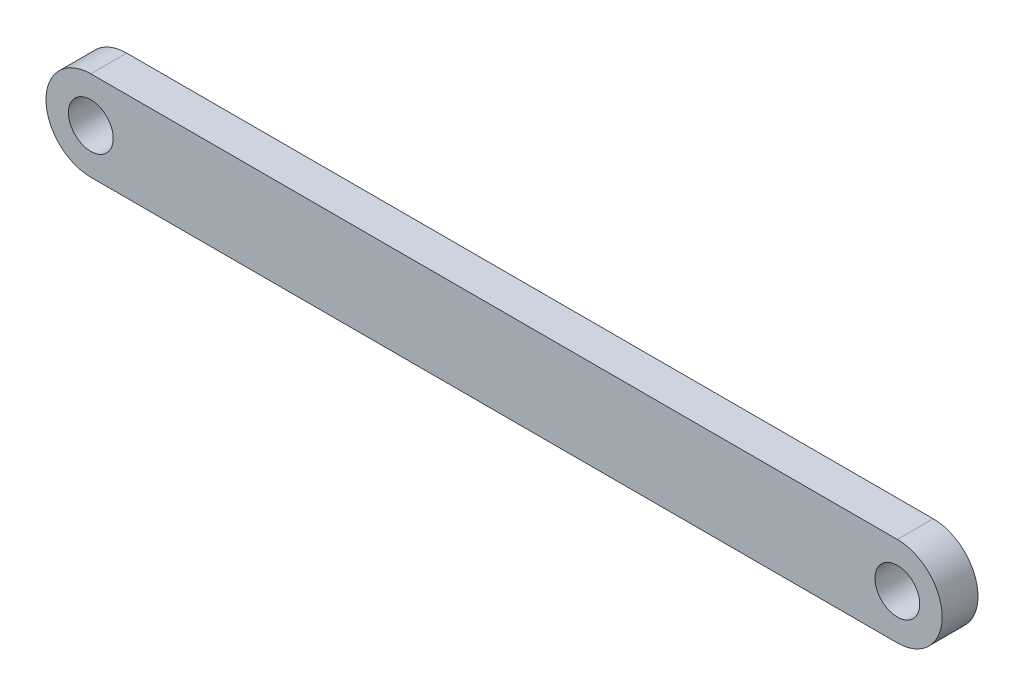
ISO-10303-21;
HEADER;
FILE_DESCRIPTION(('STEP AP214'),'2;1');
FILE_NAME('part.step','',(''),(''),'','','');
FILE_SCHEMA(('AUTOMOTIVE_DESIGN { 1 0 10303 214 1 1 1 1 }'));
ENDSEC;
DATA;
#1=APPLICATION_CONTEXT('core data for automotive mechanical design processes');
#2=APPLICATION_PROTOCOL_DEFINITION('international standard','automotive_design',2000,#1);
#3=PRODUCT_CONTEXT('',#1,'mechanical');
#4=PRODUCT('Part','Part','',(#3));
#5=PRODUCT_RELATED_PRODUCT_CATEGORY('part','',(#4));
#6=PRODUCT_DEFINITION_FORMATION('','',#4);
#7=PRODUCT_DEFINITION_CONTEXT('part definition',#1,'design');
#8=PRODUCT_DEFINITION('design','',#6,#7);
#9=PRODUCT_DEFINITION_SHAPE('','',#8);
#10=(LENGTH_UNIT() NAMED_UNIT(*) SI_UNIT(.MILLI.,.METRE.));
#11=(NAMED_UNIT(*) PLANE_ANGLE_UNIT() SI_UNIT($,.RADIAN.));
#12=(NAMED_UNIT(*) SI_UNIT($,.STERADIAN.) SOLID_ANGLE_UNIT());
#13=UNCERTAINTY_MEASURE_WITH_UNIT(LENGTH_MEASURE(1.E-05),#10,'distance_accuracy_value','');
#14=(GEOMETRIC_REPRESENTATION_CONTEXT(3) GLOBAL_UNCERTAINTY_ASSIGNED_CONTEXT((#13)) GLOBAL_UNIT_ASSIGNED_CONTEXT((#10,
#11,#12)) REPRESENTATION_CONTEXT('',''));
#15=CARTESIAN_POINT('',(0.,0.,0.));
#16=DIRECTION('',(0.,0.,1.));
#17=DIRECTION('',(1.,0.,0.));
#18=AXIS2_PLACEMENT_3D('',#15,#16,#17);
#19=CARTESIAN_POINT('',(-45.,0.,2.));
#20=DIRECTION('',(0.,0.,1.));
#21=DIRECTION('',(1.,0.,0.));
#22=AXIS2_PLACEMENT_3D('',#19,#20,#21);
#23=PLANE('',#22);
#24=CARTESIAN_POINT('',(-45.,0.,2.));
#25=DIRECTION('',(0.,0.,1.));
#26=DIRECTION('',(1.,0.,0.));
#27=AXIS2_PLACEMENT_3D('',#24,#25,#26);
#28=CIRCLE('',#27,2.5);
#29=CARTESIAN_POINT('',(-42.5,0.,2.));
#30=VERTEX_POINT('',#29);
#31=EDGE_CURVE('E106',#30,#30,#28,.T.);
#32=ORIENTED_EDGE('',*,*,#31,.F.);
#33=EDGE_LOOP('',(#32));
#34=FACE_BOUND('',#33,.T.);
#35=CARTESIAN_POINT('',(-45.,0.,2.));
#36=DIRECTION('',(0.,0.,1.));
#37=DIRECTION('',(1.,0.,0.));
#38=AXIS2_PLACEMENT_3D('',#35,#36,#37);
#39=CIRCLE('',#38,5.);
#40=CARTESIAN_POINT('',(-45.,5.,2.));
#41=VERTEX_POINT('',#40);
#42=CARTESIAN_POINT('',(-45.,-5.,2.));
#43=VERTEX_POINT('',#42);
#44=EDGE_CURVE('E93',#41,#43,#39,.T.);
#45=ORIENTED_EDGE('',*,*,#44,.T.);
#46=DIRECTION('',(1.,0.,0.));
#47=VECTOR('',#46,1.);
#48=CARTESIAN_POINT('',(-45.,-5.,2.));
#49=LINE('',#48,#47);
#50=CARTESIAN_POINT('',(45.,-5.,2.));
#51=VERTEX_POINT('',#50);
#52=EDGE_CURVE('E88',#43,#51,#49,.T.);
#53=ORIENTED_EDGE('',*,*,#52,.T.);
#54=CARTESIAN_POINT('',(45.,0.,2.));
#55=DIRECTION('',(0.,0.,1.));
#56=DIRECTION('',(1.,0.,0.));
#57=AXIS2_PLACEMENT_3D('',#54,#55,#56);
#58=CIRCLE('',#57,5.);
#59=CARTESIAN_POINT('',(45.,5.00000000000002,2.));
#60=VERTEX_POINT('',#59);
#61=EDGE_CURVE('E90',#51,#60,#58,.T.);
#62=ORIENTED_EDGE('',*,*,#61,.T.);
#63=DIRECTION('',(-1.,0.,0.));
#64=VECTOR('',#63,1.);
#65=CARTESIAN_POINT('',(-45.,5.,2.));
#66=LINE('',#65,#64);
#67=EDGE_CURVE('E57',#60,#41,#66,.T.);
#68=ORIENTED_EDGE('',*,*,#67,.T.);
#69=EDGE_LOOP('',(#45,#53,#62,#68));
#70=FACE_BOUND('',#69,.T.);
#71=CARTESIAN_POINT('',(45.,0.,2.));
#72=DIRECTION('',(0.,0.,1.));
#73=DIRECTION('',(1.,0.,0.));
#74=AXIS2_PLACEMENT_3D('',#71,#72,#73);
#75=CIRCLE('',#74,2.5);
#76=CARTESIAN_POINT('',(47.5,0.,2.));
#77=VERTEX_POINT('',#76);
#78=EDGE_CURVE('E122',#77,#77,#75,.T.);
#79=ORIENTED_EDGE('',*,*,#78,.F.);
#80=EDGE_LOOP('',(#79));
#81=FACE_BOUND('',#80,.T.);
#82=ADVANCED_FACE('F39',(#34,#70,#81),#23,.T.);
#83=CARTESIAN_POINT('',(-45.,0.,-2.));
#84=DIRECTION('',(0.,0.,1.));
#85=DIRECTION('',(1.,0.,0.));
#86=AXIS2_PLACEMENT_3D('',#83,#84,#85);
#87=PLANE('',#86);
#88=CARTESIAN_POINT('',(-45.,0.,-2.));
#89=DIRECTION('',(0.,0.,1.));
#90=DIRECTION('',(1.,0.,0.));
#91=AXIS2_PLACEMENT_3D('',#88,#89,#90);
#92=CIRCLE('',#91,5.);
#93=CARTESIAN_POINT('',(-45.,5.,-2.));
#94=VERTEX_POINT('',#93);
#95=CARTESIAN_POINT('',(-45.,-5.,-2.));
#96=VERTEX_POINT('',#95);
#97=EDGE_CURVE('E103',#94,#96,#92,.T.);
#98=ORIENTED_EDGE('',*,*,#97,.F.);
#99=DIRECTION('',(-1.,0.,0.));
#100=VECTOR('',#99,1.);
#101=CARTESIAN_POINT('',(-45.,5.,-2.));
#102=LINE('',#101,#100);
#103=CARTESIAN_POINT('',(45.,5.00000000000002,-2.));
#104=VERTEX_POINT('',#103);
#105=EDGE_CURVE('E76',#104,#94,#102,.T.);
#106=ORIENTED_EDGE('',*,*,#105,.F.);
#107=CARTESIAN_POINT('',(45.,0.,-2.));
#108=DIRECTION('',(0.,0.,1.));
#109=DIRECTION('',(1.,0.,0.));
#110=AXIS2_PLACEMENT_3D('',#107,#108,#109);
#111=CIRCLE('',#110,5.);
#112=CARTESIAN_POINT('',(45.,-5.,-2.));
#113=VERTEX_POINT('',#112);
#114=EDGE_CURVE('E71',#113,#104,#111,.T.);
#115=ORIENTED_EDGE('',*,*,#114,.F.);
#116=DIRECTION('',(1.,0.,0.));
#117=VECTOR('',#116,1.);
#118=CARTESIAN_POINT('',(-45.,-5.,-2.));
#119=LINE('',#118,#117);
#120=EDGE_CURVE('E92',#96,#113,#119,.T.);
#121=ORIENTED_EDGE('',*,*,#120,.F.);
#122=EDGE_LOOP('',(#98,#106,#115,#121));
#123=FACE_BOUND('',#122,.T.);
#124=CARTESIAN_POINT('',(-45.,0.,-2.));
#125=DIRECTION('',(0.,0.,1.));
#126=DIRECTION('',(1.,0.,0.));
#127=AXIS2_PLACEMENT_3D('',#124,#125,#126);
#128=CIRCLE('',#127,2.5);
#129=CARTESIAN_POINT('',(-42.5,0.,-2.));
#130=VERTEX_POINT('',#129);
#131=EDGE_CURVE('E119',#130,#130,#128,.T.);
#132=ORIENTED_EDGE('',*,*,#131,.T.);
#133=EDGE_LOOP('',(#132));
#134=FACE_BOUND('',#133,.T.);
#135=CARTESIAN_POINT('',(45.,0.,-2.));
#136=DIRECTION('',(0.,0.,1.));
#137=DIRECTION('',(1.,0.,0.));
#138=AXIS2_PLACEMENT_3D('',#135,#136,#137);
#139=CIRCLE('',#138,2.5);
#140=CARTESIAN_POINT('',(47.5,0.,-2.));
#141=VERTEX_POINT('',#140);
#142=EDGE_CURVE('E121',#141,#141,#139,.T.);
#143=ORIENTED_EDGE('',*,*,#142,.T.);
#144=EDGE_LOOP('',(#143));
#145=FACE_BOUND('',#144,.T.);
#146=ADVANCED_FACE('F111',(#123,#134,#145),#87,.F.);
#147=CARTESIAN_POINT('',(-45.,0.,2.));
#148=DIRECTION('',(0.,0.,-1.));
#149=DIRECTION('',(-1.,0.,0.));
#150=AXIS2_PLACEMENT_3D('',#147,#148,#149);
#151=CYLINDRICAL_SURFACE('',#150,5.);
#152=ORIENTED_EDGE('',*,*,#97,.T.);
#153=DIRECTION('',(0.,0.,-1.));
#154=VECTOR('',#153,1.);
#155=CARTESIAN_POINT('',(-45.,-5.,2.));
#156=LINE('',#155,#154);
#157=EDGE_CURVE('E11',#43,#96,#156,.T.);
#158=ORIENTED_EDGE('',*,*,#157,.F.);
#159=ORIENTED_EDGE('',*,*,#44,.F.);
#160=DIRECTION('',(0.,0.,-1.));
#161=VECTOR('',#160,1.);
#162=CARTESIAN_POINT('',(-45.,5.,2.));
#163=LINE('',#162,#161);
#164=EDGE_CURVE('E97',#41,#94,#163,.T.);
#165=ORIENTED_EDGE('',*,*,#164,.T.);
#166=EDGE_LOOP('',(#152,#158,#159,#165));
#167=FACE_BOUND('',#166,.T.);
#168=ADVANCED_FACE('F41',(#167),#151,.T.);
#169=CARTESIAN_POINT('',(-45.,-5.,2.));
#170=DIRECTION('',(0.,1.,0.));
#171=DIRECTION('',(-1.,0.,0.));
#172=AXIS2_PLACEMENT_3D('',#169,#170,#171);
#173=PLANE('',#172);
#174=ORIENTED_EDGE('',*,*,#120,.T.);
#175=DIRECTION('',(0.,0.,-1.));
#176=VECTOR('',#175,1.);
#177=CARTESIAN_POINT('',(45.,-5.,2.));
#178=LINE('',#177,#176);
#179=EDGE_CURVE('E48',#51,#113,#178,.T.);
#180=ORIENTED_EDGE('',*,*,#179,.F.);
#181=ORIENTED_EDGE('',*,*,#52,.F.);
#182=ORIENTED_EDGE('',*,*,#157,.T.);
#183=EDGE_LOOP('',(#174,#180,#181,#182));
#184=FACE_BOUND('',#183,.T.);
#185=ADVANCED_FACE('F94',(#184),#173,.F.);
#186=CARTESIAN_POINT('',(45.,0.,2.));
#187=DIRECTION('',(0.,0.,-1.));
#188=DIRECTION('',(-1.,0.,0.));
#189=AXIS2_PLACEMENT_3D('',#186,#187,#188);
#190=CYLINDRICAL_SURFACE('',#189,5.);
#191=ORIENTED_EDGE('',*,*,#114,.T.);
#192=DIRECTION('',(0.,0.,-1.));
#193=VECTOR('',#192,1.);
#194=CARTESIAN_POINT('',(45.,5.00000000000002,2.));
#195=LINE('',#194,#193);
#196=EDGE_CURVE('E96',#60,#104,#195,.T.);
#197=ORIENTED_EDGE('',*,*,#196,.F.);
#198=ORIENTED_EDGE('',*,*,#61,.F.);
#199=ORIENTED_EDGE('',*,*,#179,.T.);
#200=EDGE_LOOP('',(#191,#197,#198,#199));
#201=FACE_BOUND('',#200,.T.);
#202=ADVANCED_FACE('F100',(#201),#190,.T.);
#203=CARTESIAN_POINT('',(-45.,5.,2.));
#204=DIRECTION('',(0.,-1.,0.));
#205=DIRECTION('',(1.,0.,0.));
#206=AXIS2_PLACEMENT_3D('',#203,#204,#205);
#207=PLANE('',#206);
#208=ORIENTED_EDGE('',*,*,#105,.T.);
#209=ORIENTED_EDGE('',*,*,#164,.F.);
#210=ORIENTED_EDGE('',*,*,#67,.F.);
#211=ORIENTED_EDGE('',*,*,#196,.T.);
#212=EDGE_LOOP('',(#208,#209,#210,#211));
#213=FACE_BOUND('',#212,.T.);
#214=ADVANCED_FACE('F112',(#213),#207,.F.);
#215=CARTESIAN_POINT('',(-45.,0.,2.));
#216=DIRECTION('',(0.,0.,-1.));
#217=DIRECTION('',(-1.,0.,0.));
#218=AXIS2_PLACEMENT_3D('',#215,#216,#217);
#219=CYLINDRICAL_SURFACE('',#218,2.5);
#220=ORIENTED_EDGE('',*,*,#31,.T.);
#221=EDGE_LOOP('',(#220));
#222=FACE_BOUND('',#221,.T.);
#223=ORIENTED_EDGE('',*,*,#131,.F.);
#224=EDGE_LOOP('',(#223));
#225=FACE_BOUND('',#224,.T.);
#226=ADVANCED_FACE('F143',(#222,#225),#219,.F.);
#227=CARTESIAN_POINT('',(45.,0.,2.));
#228=DIRECTION('',(0.,0.,-1.));
#229=DIRECTION('',(-1.,0.,0.));
#230=AXIS2_PLACEMENT_3D('',#227,#228,#229);
#231=CYLINDRICAL_SURFACE('',#230,2.5);
#232=ORIENTED_EDGE('',*,*,#78,.T.);
#233=EDGE_LOOP('',(#232));
#234=FACE_BOUND('',#233,.T.);
#235=ORIENTED_EDGE('',*,*,#142,.F.);
#236=EDGE_LOOP('',(#235));
#237=FACE_BOUND('',#236,.T.);
#238=ADVANCED_FACE('F128',(#234,#237),#231,.F.);
#239=CLOSED_SHELL('',(#82,#146,#168,#185,#202,#214,#226,#238));
#240=MANIFOLD_SOLID_BREP('B2',#239);
#241=ADVANCED_BREP_SHAPE_REPRESENTATION('',(#18,#240),#14);
#242=SHAPE_DEFINITION_REPRESENTATION(#9,#241);
ENDSEC;
END-ISO-10303-21;
